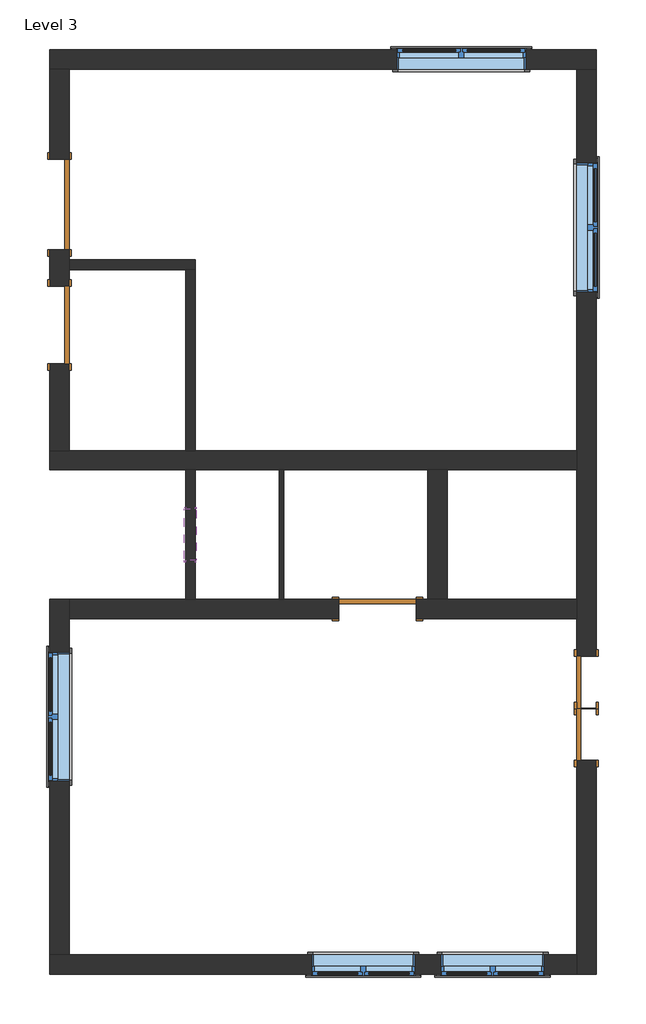
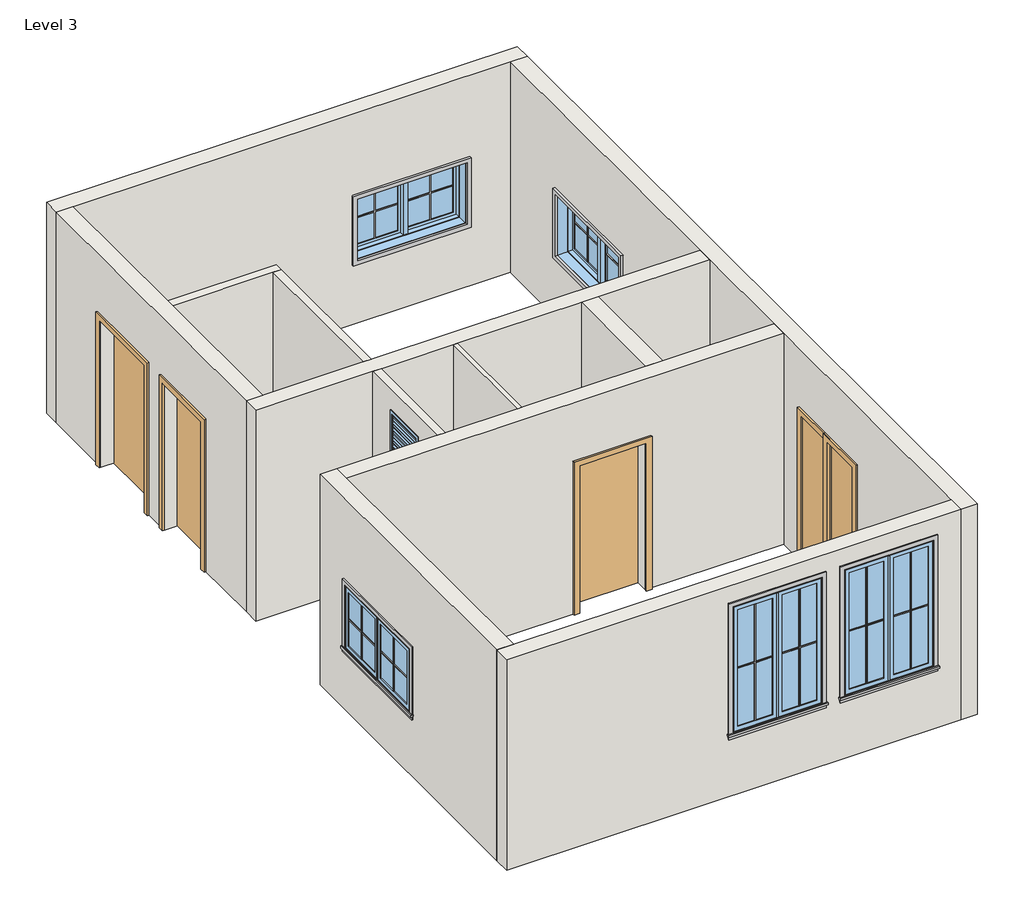
# One storey: 20 proxies, 12 walls, 6 windows, 5 doors.
"""IFC4 building model written with IfcOpenShell, lengths in millimetres."""

from ifc_helpers import new_model, si_unit, frame, origin, place, context, project, spatial, polyline, outline, extrude, faceted_brep, transform, mapped, element, save
from components import muntin_pattern_2x2_muntin_pattern_2x2_9352d081, muntin_pattern_2x2_muntin_pattern_2x2_5c2cbe28, muntin_pattern_2x2_muntin_pattern_2x2_2b4d9f72, muntin_pattern_2x2_muntin_pattern_2x2_ef995ed3, trim_window_exterior_flat_with_sill_979bde60, trim_window_exterior_flat_with_sill_b7e4d11c, trim_window_interior_flat_picture_frame_7883d11b, trim_window_interior_flat_picture_frame_936b8d2a, single_flush_door_2_0d3b4037, single_flush_door_2_4a3212df, door_a90ba1ad, door_0ca8825f, door_9d399b00, window_casement_double_c1d95f0f, window_casement_double_wall_4_6ca1769e, window_d39e7ecb

model = new_model("IFC4")

# Units and contexts
model_context = context("Model", 3, world=origin())
ifc_project = project(units=[si_unit("LENGTHUNIT", "METRE", prefix="MILLI")], contexts=[model_context])

# Site, building, storey
site = spatial("IfcSite", under=ifc_project)
building = spatial("IfcBuilding", under=site)
storey = spatial("IfcBuildingStorey", under=building, Name="Level 3", Elevation=3200.4)

# Proxies
placement = place(None, origin())
muntin_pattern_2x2_muntin_pattern_2x2_shape = muntin_pattern_2x2_muntin_pattern_2x2_9352d081(model_context)
element("IfcBuildingElementProxy", 1, Name="Muntin Pattern_2x2 : Muntin Pattern_2x2", ObjectType="Muntin Pattern_2x2 : Muntin Pattern_2x2", at=placement, inside=storey, context=model_context, shape_type="MappedRepresentation", body=[
    mapped(muntin_pattern_2x2_muntin_pattern_2x2_shape, transform((-4785.3510342, -2707.8617544, 4184.65), x_axis=(0.0, 1.0, 0.0), y_axis=(-1.0, 0.0, 0.0), z_axis=(0.0, 0.0, 1.0))),
])
element("IfcBuildingElementProxy", 2, Name="Muntin Pattern_2x2 : Muntin Pattern_2x2", ObjectType="Muntin Pattern_2x2 : Muntin Pattern_2x2", at=placement, inside=storey, context=model_context, shape_type="MappedRepresentation", body=[
    mapped(muntin_pattern_2x2_muntin_pattern_2x2_shape, transform((1634.4989658, 3816.7632456, 4184.65), x_axis=(0.0, -1.0, 0.0), y_axis=(1.0, 0.0, 0.0), z_axis=(0.0, 0.0, 1.0))),
])
element("IfcBuildingElementProxy", 3, Name="Muntin Pattern_2x2 : Muntin Pattern_2x2", ObjectType="Muntin Pattern_2x2 : Muntin Pattern_2x2", at=placement, inside=storey, context=model_context, shape_type="MappedRepresentation", body=[
    mapped(muntin_pattern_2x2_muntin_pattern_2x2_shape, transform((-322.8885342, 5523.3257456, 4184.65), x_axis=(1.0, 0.0, 0.0), y_axis=(0.0, 1.0, 0.0), z_axis=(0.0, 0.0, 1.0))),
])
muntin_pattern_2x2_muntin_pattern_2x2_2_shape = muntin_pattern_2x2_muntin_pattern_2x2_5c2cbe28(model_context)
element("IfcBuildingElementProxy", 4, Name="Muntin Pattern_2x2 : Muntin Pattern_2x2", ObjectType="Muntin Pattern_2x2 : Muntin Pattern_2x2", at=placement, inside=storey, context=model_context, shape_type="MappedRepresentation", body=[
    mapped(muntin_pattern_2x2_muntin_pattern_2x2_2_shape, transform((-4785.3510342, -1949.0367544, 4184.65), x_axis=(0.0, -1.0, 0.0), y_axis=(1.0, 0.0, 0.0), z_axis=(0.0, 0.0, 1.0))),
])
element("IfcBuildingElementProxy", 5, Name="Muntin Pattern_2x2 : Muntin Pattern_2x2", ObjectType="Muntin Pattern_2x2 : Muntin Pattern_2x2", at=placement, inside=storey, context=model_context, shape_type="MappedRepresentation", body=[
    mapped(muntin_pattern_2x2_muntin_pattern_2x2_2_shape, transform((1634.4989658, 3057.9382456, 4184.65), x_axis=(0.0, 1.0, 0.0), y_axis=(-1.0, 0.0, 0.0), z_axis=(0.0, 0.0, 1.0))),
])
element("IfcBuildingElementProxy", 6, Name="Muntin Pattern_2x2 : Muntin Pattern_2x2", ObjectType="Muntin Pattern_2x2 : Muntin Pattern_2x2", at=placement, inside=storey, context=model_context, shape_type="MappedRepresentation", body=[
    mapped(muntin_pattern_2x2_muntin_pattern_2x2_2_shape, transform((435.9364658, 5523.3257456, 4184.65), x_axis=(-1.0, 0.0, 0.0), y_axis=(0.0, -1.0, 0.0), z_axis=(0.0, 0.0, 1.0))),
])
muntin_pattern_2x2_muntin_pattern_2x2_3_shape = muntin_pattern_2x2_muntin_pattern_2x2_2b4d9f72(model_context)
element("IfcBuildingElementProxy", 7, Name="Muntin Pattern_2x2 : Muntin Pattern_2x2", ObjectType="Muntin Pattern_2x2 : Muntin Pattern_2x2", at=placement, inside=storey, context=model_context, shape_type="MappedRepresentation", body=[
    mapped(muntin_pattern_2x2_muntin_pattern_2x2_3_shape, transform((-795.9635342, -5354.2242544, 4184.65), x_axis=(-1.0, 0.0, 0.0), y_axis=(0.0, -1.0, 0.0), z_axis=(0.0, 0.0, 1.0))),
])
element("IfcBuildingElementProxy", 8, Name="Muntin Pattern_2x2 : Muntin Pattern_2x2", ObjectType="Muntin Pattern_2x2 : Muntin Pattern_2x2", at=placement, inside=storey, context=model_context, shape_type="MappedRepresentation", body=[
    mapped(muntin_pattern_2x2_muntin_pattern_2x2_3_shape, transform((728.0364658, -5354.2242544, 4184.65), x_axis=(-1.0, 0.0, 0.0), y_axis=(0.0, -1.0, 0.0), z_axis=(0.0, 0.0, 1.0))),
])
muntin_pattern_2x2_muntin_pattern_2x2_4_shape = muntin_pattern_2x2_muntin_pattern_2x2_ef995ed3(model_context)
element("IfcBuildingElementProxy", 9, Name="Muntin Pattern_2x2 : Muntin Pattern_2x2", ObjectType="Muntin Pattern_2x2 : Muntin Pattern_2x2", at=placement, inside=storey, context=model_context, shape_type="MappedRepresentation", body=[
    mapped(muntin_pattern_2x2_muntin_pattern_2x2_4_shape, transform((-1402.3885342, -5354.2242544, 4184.65), x_axis=(1.0, 0.0, 0.0), y_axis=(0.0, 1.0, 0.0), z_axis=(0.0, 0.0, 1.0))),
])
element("IfcBuildingElementProxy", 10, Name="Muntin Pattern_2x2 : Muntin Pattern_2x2", ObjectType="Muntin Pattern_2x2 : Muntin Pattern_2x2", at=placement, inside=storey, context=model_context, shape_type="MappedRepresentation", body=[
    mapped(muntin_pattern_2x2_muntin_pattern_2x2_4_shape, transform((121.6114658, -5354.2242544, 4184.65), x_axis=(1.0, 0.0, 0.0), y_axis=(0.0, 1.0, 0.0), z_axis=(0.0, 0.0, 1.0))),
])
trim_window_exterior_flat_with_sill_shape = trim_window_exterior_flat_with_sill_979bde60(model_context)
element("IfcBuildingElementProxy", 11, Name="Trim-Window-Exterior-Flat : with Sill", ObjectType="Trim-Window-Exterior-Flat : with Sill", at=placement, inside=storey, context=model_context, shape_type="MappedRepresentation", body=[
    mapped(trim_window_exterior_flat_with_sill_shape, transform((-4794.8760342, -2328.4492544, 5029.2), x_axis=(0.0, -1.0, 0.0), y_axis=(0.0, 0.0, 1.0), z_axis=(-1.0, 0.0, 0.0))),
])
element("IfcBuildingElementProxy", 12, Name="Trim-Window-Exterior-Flat : with Sill", ObjectType="Trim-Window-Exterior-Flat : with Sill", at=placement, inside=storey, context=model_context, shape_type="MappedRepresentation", body=[
    mapped(trim_window_exterior_flat_with_sill_shape, transform((1644.0239658, 3437.3507456, 5029.2), x_axis=(0.0, 1.0, 0.0), y_axis=(0.0, 0.0, 1.0), z_axis=(1.0, 0.0, 0.0))),
])
element("IfcBuildingElementProxy", 13, Name="Trim-Window-Exterior-Flat : with Sill", ObjectType="Trim-Window-Exterior-Flat : with Sill", at=placement, inside=storey, context=model_context, shape_type="MappedRepresentation", body=[
    mapped(trim_window_exterior_flat_with_sill_shape, transform((56.5239658, 5532.8507456, 5029.2), x_axis=(-1.0, 0.0, 0.0), y_axis=(0.0, 0.0, 1.0), z_axis=(0.0, 1.0, 0.0))),
])
trim_window_exterior_flat_with_sill_2_shape = trim_window_exterior_flat_with_sill_b7e4d11c(model_context)
element("IfcBuildingElementProxy", 14, Name="Trim-Window-Exterior-Flat : with Sill", ObjectType="Trim-Window-Exterior-Flat : with Sill", at=placement, inside=storey, context=model_context, shape_type="MappedRepresentation", body=[
    mapped(trim_window_exterior_flat_with_sill_2_shape, transform((-1099.1760342, -5363.7492544, 5943.6), x_axis=(1.0, 0.0, 0.0), y_axis=(0.0, 0.0, 1.0), z_axis=(0.0, -1.0, 0.0))),
])
element("IfcBuildingElementProxy", 15, Name="Trim-Window-Exterior-Flat : with Sill", ObjectType="Trim-Window-Exterior-Flat : with Sill", at=placement, inside=storey, context=model_context, shape_type="MappedRepresentation", body=[
    mapped(trim_window_exterior_flat_with_sill_2_shape, transform((424.8239658, -5363.7492544, 5943.6), x_axis=(1.0, 0.0, 0.0), y_axis=(0.0, 0.0, 1.0), z_axis=(0.0, -1.0, 0.0))),
])
trim_window_interior_flat_picture_frame_shape = trim_window_interior_flat_picture_frame_7883d11b(model_context)
element("IfcBuildingElementProxy", 16, Name="Trim-Window-Interior-Flat : Picture Frame", ObjectType="Trim-Window-Interior-Flat : Picture Frame", at=placement, inside=storey, context=model_context, shape_type="MappedRepresentation", body=[
    mapped(trim_window_interior_flat_picture_frame_shape, transform((-4566.2760342, -2328.4492544, 5029.2), x_axis=(0.0, 1.0, 0.0), y_axis=(0.0, 0.0, 1.0), z_axis=(1.0, 0.0, 0.0))),
])
element("IfcBuildingElementProxy", 17, Name="Trim-Window-Interior-Flat : Picture Frame", ObjectType="Trim-Window-Interior-Flat : Picture Frame", at=placement, inside=storey, context=model_context, shape_type="MappedRepresentation", body=[
    mapped(trim_window_interior_flat_picture_frame_shape, transform((1415.4239658, 3437.3507456, 5029.2), x_axis=(0.0, -1.0, 0.0), y_axis=(0.0, 0.0, 1.0), z_axis=(-1.0, 0.0, 0.0))),
])
element("IfcBuildingElementProxy", 18, Name="Trim-Window-Interior-Flat : Picture Frame", ObjectType="Trim-Window-Interior-Flat : Picture Frame", at=placement, inside=storey, context=model_context, shape_type="MappedRepresentation", body=[
    mapped(trim_window_interior_flat_picture_frame_shape, transform((56.5239658, 5304.2507456, 5029.2), x_axis=(1.0, 0.0, 0.0), y_axis=(0.0, 0.0, 1.0), z_axis=(0.0, -1.0, 0.0))),
])
trim_window_interior_flat_picture_frame_2_shape = trim_window_interior_flat_picture_frame_936b8d2a(model_context)
element("IfcBuildingElementProxy", 19, Name="Trim-Window-Interior-Flat : Picture Frame", ObjectType="Trim-Window-Interior-Flat : Picture Frame", at=placement, inside=storey, context=model_context, shape_type="MappedRepresentation", body=[
    mapped(trim_window_interior_flat_picture_frame_2_shape, transform((-1099.1760342, -5135.1492544, 5943.6), x_axis=(-1.0, 0.0, 0.0), y_axis=(0.0, 0.0, 1.0), z_axis=(0.0, 1.0, 0.0))),
])
element("IfcBuildingElementProxy", 20, Name="Trim-Window-Interior-Flat : Picture Frame", ObjectType="Trim-Window-Interior-Flat : Picture Frame", at=placement, inside=storey, context=model_context, shape_type="MappedRepresentation", body=[
    mapped(trim_window_interior_flat_picture_frame_2_shape, transform((424.8239658, -5135.1492544, 5943.6), x_axis=(-1.0, 0.0, 0.0), y_axis=(0.0, 0.0, 1.0), z_axis=(0.0, 1.0, 0.0))),
])

# Doors
single_flush_door_2_shape = single_flush_door_2_0d3b4037(model_context)
element("IfcDoor", 21, ObjectType="Single-Flush : door 2'", at=placement, inside=storey, context=model_context, shape_type="MappedRepresentation", body=[
    mapped(single_flush_door_2_shape, transform((1529.7239658, -1922.0492544, 3200.4), x_axis=(0.0, 1.0, 0.0), y_axis=(-1.0, 0.0, 0.0), z_axis=(0.0, 0.0, 1.0))),
])
single_flush_door_2_2_shape = single_flush_door_2_4a3212df(model_context)
element("IfcDoor", 22, ObjectType="Single-Flush : door 2'", at=placement, inside=storey, context=model_context, shape_type="MappedRepresentation", body=[
    mapped(single_flush_door_2_2_shape, transform((1529.7239658, -2537.9992544, 3200.4), x_axis=(0.0, -1.0, 0.0), y_axis=(1.0, 0.0, 0.0), z_axis=(0.0, 0.0, 1.0))),
])
door_shape = door_a90ba1ad(model_context)
element("IfcDoor", 23, ObjectType="Single-Flush : door 2'6\"", at=placement, inside=storey, context=model_context, shape_type="MappedRepresentation", body=[
    mapped(door_shape, transform((-4680.5760342, 2288.0007456, 3200.4), x_axis=(0.0, 1.0, 0.0), y_axis=(-1.0, 0.0, 0.0), z_axis=(0.0, 0.0, 1.0))),
])
door_2_shape = door_0ca8825f(model_context)
element("IfcDoor", 24, ObjectType="Single-Flush : door 2'6\"", at=placement, inside=storey, context=model_context, shape_type="MappedRepresentation", body=[
    mapped(door_2_shape, transform((-934.0760342, -1058.4492544, 3200.4), x_axis=(1.0, 0.0, 0.0), y_axis=(0.0, 1.0, 0.0), z_axis=(0.0, 0.0, 1.0))),
])
door_3_shape = door_9d399b00(model_context)
element("IfcDoor", 25, ObjectType="Single-Flush : door 3'6\"", at=placement, inside=storey, context=model_context, shape_type="MappedRepresentation", body=[
    mapped(door_3_shape, transform((-4680.5760342, 3710.4007456, 3200.4), x_axis=(0.0, -1.0, 0.0), y_axis=(1.0, 0.0, 0.0), z_axis=(0.0, 0.0, 1.0))),
])

# Walls
element("IfcWall", 26, ObjectType="wall 2\"", at=placement, inside=storey, context=model_context, shape_type="SweptSolid", body=[
    extrude(outline(polyline([(-2089.7760342, -944.1492544), (-2089.7760342, 579.8507456), (-2038.9760342, 579.8507456), (-2038.9760342, -944.1492544), (-2089.7760342, -944.1492544)])), frame((0.0, 0.0, 3200.4), z_axis=(0.0, 0.0, 1.0), x_axis=(1.0, 0.0, 0.0)), (0.0, 0.0, 1.0), 3048.0),
])
element("IfcWall", 27, ObjectType="wall 4.5\"", at=placement, inside=storey, context=model_context, shape_type="Brep", body=[
    faceted_brep([(-4566.2760342, 2942.0507456, 3200.4), (-3194.6760342, 2942.0507456, 3200.4), (-3080.3760342, 2942.0507456, 3200.4), (-3080.3760342, 2942.0507456, 6248.4), (-3194.6760342, 2942.0507456, 6248.4), (-4566.2760342, 2942.0507456, 6248.4), (-4566.2760342, 3056.3507456, 3200.4), (-4566.2760342, 3056.3507456, 6248.4), (-3080.3760342, 3056.3507456, 6248.4), (-3080.3760342, 3056.3507456, 3200.4)], [[[0, 1, 2, 3, 4, 5]], [[6, 7, 8, 9]], [[2, 1, 0, 6, 9]], [[0, 5, 7, 6]], [[3, 2, 9, 8]], [[5, 4, 3, 8, 7]]]),
])
element("IfcWall", 28, ObjectType="wall 4.5\"", at=placement, inside=storey, context=model_context, shape_type="SweptSolid", body=[
    extrude(outline(polyline([(-3194.6760342, 808.4507456), (-3194.6760342, 2942.0507456), (-3080.3760342, 2942.0507456), (-3080.3760342, 808.4507456), (-3194.6760342, 808.4507456)])), frame((0.0, 0.0, 3200.4), z_axis=(0.0, 0.0, 1.0), x_axis=(1.0, 0.0, 0.0)), (0.0, 0.0, 1.0), 3048.0),
])
element("IfcWall", 29, ObjectType="wall 4.5\"", at=placement, inside=storey, context=model_context, shape_type="SweptSolid", body=[
    extrude(outline(polyline([(579.8507456, 3200.4), (-944.1492544, 3200.4), (-944.1492544, 6248.4), (579.8507456, 6248.4), (579.8507456, 3200.4)]), holes=[polyline([(-486.9492544, 5943.6), (-486.9492544, 5334.0), (122.6507456, 5334.0), (122.6507456, 5943.6), (-486.9492544, 5943.6)])]), frame((-3194.6760342, 0.0, 0.0), z_axis=(1.0, 0.0, 0.0), x_axis=(0.0, 1.0, 0.0)), (0.0, 0.0, 1.0), 114.3),
])
element("IfcWall", 30, ObjectType="wall 9\"", at=placement, inside=storey, context=model_context, shape_type="Brep", body=[
    faceted_brep([(-4794.8760342, 5304.2507456, 3200.4), (-4566.2760342, 5304.2507456, 3200.4), (1415.4239658, 5304.2507456, 3200.4), (1644.0239658, 5304.2507456, 3200.4), (1644.0239658, 5304.2507456, 6248.4), (1415.4239658, 5304.2507456, 6248.4), (-4566.2760342, 5304.2507456, 6248.4), (-4794.8760342, 5304.2507456, 6248.4), (818.5239658, 5304.2507456, 5029.2), (818.5239658, 5304.2507456, 4114.8), (-705.4760342, 5304.2507456, 4114.8), (-705.4760342, 5304.2507456, 5029.2), (-4794.8760342, 5532.8507456, 3200.4), (-4794.8760342, 5532.8507456, 6248.4), (1644.0239658, 5532.8507456, 6248.4), (1644.0239658, 5532.8507456, 3200.4), (818.5239658, 5532.8507456, 5029.2), (-705.4760342, 5532.8507456, 5029.2), (-705.4760342, 5532.8507456, 4114.8), (818.5239658, 5532.8507456, 4114.8)], [[[0, 1, 2, 3, 4, 5, 6, 7], [8, 9, 10, 11]], [[12, 13, 14, 15], [16, 17, 18, 19]], [[3, 2, 1, 0, 12, 15]], [[4, 3, 15, 14]], [[0, 7, 13, 12]], [[9, 8, 16, 19]], [[10, 9, 19, 18]], [[11, 10, 18, 17]], [[8, 11, 17, 16]], [[7, 6, 5, 4, 14, 13]]]),
])
element("IfcWall", 31, ObjectType="wall 9\"", at=placement, inside=storey, context=model_context, shape_type="Brep", body=[
    faceted_brep([(1415.4239658, 5304.2507456, 6248.4), (1415.4239658, 5304.2507456, 3200.4), (1415.4239658, 808.4507456, 3200.4), (1415.4239658, 579.8507456, 3200.4), (1415.4239658, -944.1492544, 3200.4), (1415.4239658, -1172.7492544, 3200.4), (1415.4239658, -1617.2492544, 3200.4), (1415.4239658, -1617.2492544, 5334.0), (1415.4239658, -2226.8492544, 5334.0), (1415.4239658, -2226.8492544, 3200.4), (1415.4239658, -2233.1992544, 3200.4), (1415.4239658, -2233.1992544, 5334.0), (1415.4239658, -2842.7992544, 5334.0), (1415.4239658, -2842.7992544, 3200.4), (1415.4239658, -5135.1492544, 3200.4), (1415.4239658, -5363.7492544, 3200.4), (1415.4239658, -5363.7492544, 6248.4), (1415.4239658, -5135.1492544, 6248.4), (1415.4239658, -1172.7492544, 6248.4), (1415.4239658, -944.1492544, 6248.4), (1415.4239658, 579.8507456, 6248.4), (1415.4239658, 808.4507456, 6248.4), (1415.4239658, 2675.3507456, 5029.2), (1415.4239658, 2675.3507456, 4114.8), (1415.4239658, 4199.3507456, 4114.8), (1415.4239658, 4199.3507456, 5029.2), (1644.0239658, 5304.2507456, 3200.4), (1644.0239658, 5304.2507456, 6248.4), (1644.0239658, -5363.7492544, 6248.4), (1644.0239658, -5363.7492544, 3200.4), (1644.0239658, -2842.7992544, 3200.4), (1644.0239658, -2842.7992544, 5334.0), (1644.0239658, -2233.1992544, 5334.0), (1644.0239658, -2233.1992544, 3200.4), (1644.0239658, -2226.8492544, 3200.4), (1644.0239658, -2226.8492544, 5334.0), (1644.0239658, -1617.2492544, 5334.0), (1644.0239658, -1617.2492544, 3200.4), (1644.0239658, 2675.3507456, 5029.2), (1644.0239658, 4199.3507456, 5029.2), (1644.0239658, 4199.3507456, 4114.8), (1644.0239658, 2675.3507456, 4114.8)], [[[0, 1, 2, 3, 4, 5, 6, 7, 8, 9, 10, 11, 12, 13, 14, 15, 16, 17, 18, 19, 20, 21], [22, 23, 24, 25]], [[26, 27, 28, 29, 30, 31, 32, 33, 34, 35, 36, 37], [38, 39, 40, 41]], [[1, 26, 37, 6, 5, 4, 3, 2]], [[29, 15, 14, 13, 30]], [[9, 34, 33, 10]], [[1, 0, 27, 26]], [[16, 15, 29, 28]], [[23, 22, 38, 41]], [[24, 23, 41, 40]], [[25, 24, 40, 39]], [[22, 25, 39, 38]], [[7, 6, 37, 36]], [[8, 7, 36, 35]], [[9, 8, 35, 34]], [[12, 31, 30, 13]], [[31, 12, 11, 32]], [[32, 11, 10, 33]], [[0, 21, 20, 19, 18, 17, 16, 28, 27]]]),
])
element("IfcWall", 32, ObjectType="wall 9\"", at=placement, inside=storey, context=model_context, shape_type="Brep", body=[
    faceted_brep([(1415.4239658, 808.4507456, 3200.4), (-3080.3760342, 808.4507456, 3200.4), (-3194.6760342, 808.4507456, 3200.4), (-4566.2760342, 808.4507456, 3200.4), (-4794.8760342, 808.4507456, 3200.4), (-4794.8760342, 808.4507456, 6248.4), (-4566.2760342, 808.4507456, 6248.4), (-3194.6760342, 808.4507456, 6248.4), (-3080.3760342, 808.4507456, 6248.4), (1415.4239658, 808.4507456, 6248.4), (1415.4239658, 579.8507456, 3200.4), (1415.4239658, 579.8507456, 6248.4), (-108.5760342, 579.8507456, 6248.4), (-337.1760342, 579.8507456, 6248.4), (-2038.9760342, 579.8507456, 6248.4), (-2089.7760342, 579.8507456, 6248.4), (-3080.3760342, 579.8507456, 6248.4), (-3194.6760342, 579.8507456, 6248.4), (-4794.8760342, 579.8507456, 6248.4), (-4794.8760342, 579.8507456, 3200.4), (-3194.6760342, 579.8507456, 3200.4), (-3080.3760342, 579.8507456, 3200.4), (-2089.7760342, 579.8507456, 3200.4), (-2038.9760342, 579.8507456, 3200.4), (-337.1760342, 579.8507456, 3200.4), (-108.5760342, 579.8507456, 3200.4)], [[[0, 1, 2, 3, 4, 5, 6, 7, 8, 9]], [[10, 11, 12, 13, 14, 15, 16, 17, 18, 19, 20, 21, 22, 23, 24, 25]], [[4, 3, 2, 1, 0, 10, 25, 24, 23, 22, 21, 20, 19]], [[0, 9, 11, 10]], [[5, 4, 19, 18]], [[9, 8, 7, 6, 5, 18, 17, 16, 15, 14, 13, 12, 11]]]),
])
element("IfcWall", 33, ObjectType="wall 9\"", at=placement, inside=storey, context=model_context, shape_type="Brep", body=[
    faceted_brep([(-4566.2760342, 2745.2007456, 5334.0), (-4566.2760342, 2745.2007456, 3200.4), (-4566.2760342, 2942.0507456, 3200.4), (-4566.2760342, 3056.3507456, 3200.4), (-4566.2760342, 3177.0007456, 3200.4), (-4566.2760342, 3177.0007456, 5334.0), (-4566.2760342, 4243.8007456, 5334.0), (-4566.2760342, 4243.8007456, 3200.4), (-4566.2760342, 5304.2507456, 3200.4), (-4566.2760342, 5304.2507456, 6248.4), (-4566.2760342, 3056.3507456, 6248.4), (-4566.2760342, 2942.0507456, 6248.4), (-4566.2760342, 808.4507456, 6248.4), (-4566.2760342, 808.4507456, 3200.4), (-4566.2760342, 1830.8007456, 3200.4), (-4566.2760342, 1830.8007456, 5334.0), (-4794.8760342, 3177.0007456, 3200.4), (-4794.8760342, 2745.2007456, 3200.4), (-4794.8760342, 2745.2007456, 5334.0), (-4794.8760342, 1830.8007456, 5334.0), (-4794.8760342, 1830.8007456, 3200.4), (-4794.8760342, 808.4507456, 3200.4), (-4794.8760342, 808.4507456, 6248.4), (-4794.8760342, 5304.2507456, 6248.4), (-4794.8760342, 5304.2507456, 3200.4), (-4794.8760342, 4243.8007456, 3200.4), (-4794.8760342, 4243.8007456, 5334.0), (-4794.8760342, 3177.0007456, 5334.0)], [[[0, 1, 2, 3, 4, 5, 6, 7, 8, 9, 10, 11, 12, 13, 14, 15]], [[16, 17, 18, 19, 20, 21, 22, 23, 24, 25, 26, 27]], [[25, 24, 8, 7]], [[14, 13, 21, 20]], [[4, 3, 2, 1, 17, 16]], [[9, 8, 24, 23]], [[13, 12, 22, 21]], [[5, 4, 16, 27]], [[6, 5, 27, 26]], [[7, 6, 26, 25]], [[18, 17, 1, 0]], [[19, 18, 0, 15]], [[20, 19, 15, 14]], [[12, 11, 10, 9, 23, 22]]]),
])
element("IfcWall", 34, ObjectType="wall 9\"", at=placement, inside=storey, context=model_context, shape_type="Brep", body=[
    faceted_brep([(1415.4239658, -5135.1492544, 3200.4), (-4566.2760342, -5135.1492544, 3200.4), (-4794.8760342, -5135.1492544, 3200.4), (-4794.8760342, -5135.1492544, 6248.4), (-4566.2760342, -5135.1492544, 6248.4), (1415.4239658, -5135.1492544, 6248.4), (-1708.7760342, -5135.1492544, 5943.6), (-1708.7760342, -5135.1492544, 4114.8), (-489.5760342, -5135.1492544, 4114.8), (-489.5760342, -5135.1492544, 5943.6), (-184.7760342, -5135.1492544, 5943.6), (-184.7760342, -5135.1492544, 4114.8), (1034.4239658, -5135.1492544, 4114.8), (1034.4239658, -5135.1492544, 5943.6), (1415.4239658, -5363.7492544, 3200.4), (1415.4239658, -5363.7492544, 6248.4), (-4794.8760342, -5363.7492544, 6248.4), (-4794.8760342, -5363.7492544, 3200.4), (-1708.7760342, -5363.7492544, 5943.6), (-489.5760342, -5363.7492544, 5943.6), (-489.5760342, -5363.7492544, 4114.8), (-1708.7760342, -5363.7492544, 4114.8), (-184.7760342, -5363.7492544, 5943.6), (1034.4239658, -5363.7492544, 5943.6), (1034.4239658, -5363.7492544, 4114.8), (-184.7760342, -5363.7492544, 4114.8)], [[[0, 1, 2, 3, 4, 5], [6, 7, 8, 9], [10, 11, 12, 13]], [[14, 15, 16, 17], [18, 19, 20, 21], [22, 23, 24, 25]], [[2, 1, 0, 14, 17]], [[0, 5, 15, 14]], [[3, 2, 17, 16]], [[7, 6, 18, 21]], [[8, 7, 21, 20]], [[9, 8, 20, 19]], [[6, 9, 19, 18]], [[11, 10, 22, 25]], [[12, 11, 25, 24]], [[13, 12, 24, 23]], [[10, 13, 23, 22]], [[5, 4, 3, 16, 15]]]),
])
element("IfcWall", 35, ObjectType="wall 9\"", at=placement, inside=storey, context=model_context, shape_type="Brep", body=[
    faceted_brep([(-4566.2760342, -5135.1492544, 3200.4), (-4566.2760342, -1172.7492544, 3200.4), (-4566.2760342, -944.1492544, 3200.4), (-4566.2760342, -944.1492544, 6248.4), (-4566.2760342, -1172.7492544, 6248.4), (-4566.2760342, -5135.1492544, 6248.4), (-4566.2760342, -1566.4492544, 5029.2), (-4566.2760342, -1566.4492544, 4114.8), (-4566.2760342, -3090.4492544, 4114.8), (-4566.2760342, -3090.4492544, 5029.2), (-4794.8760342, -5135.1492544, 3200.4), (-4794.8760342, -5135.1492544, 6248.4), (-4794.8760342, -944.1492544, 6248.4), (-4794.8760342, -944.1492544, 3200.4), (-4794.8760342, -1566.4492544, 5029.2), (-4794.8760342, -3090.4492544, 5029.2), (-4794.8760342, -3090.4492544, 4114.8), (-4794.8760342, -1566.4492544, 4114.8)], [[[0, 1, 2, 3, 4, 5], [6, 7, 8, 9]], [[10, 11, 12, 13], [14, 15, 16, 17]], [[2, 1, 0, 10, 13]], [[0, 5, 11, 10]], [[3, 2, 13, 12]], [[7, 6, 14, 17]], [[8, 7, 17, 16]], [[9, 8, 16, 15]], [[6, 9, 15, 14]], [[5, 4, 3, 12, 11]]]),
])
element("IfcWall", 36, ObjectType="wall 9\"", at=placement, inside=storey, context=model_context, shape_type="Brep", body=[
    faceted_brep([(-476.8760342, -1172.7492544, 5334.0), (-476.8760342, -1172.7492544, 3200.4), (1415.4239658, -1172.7492544, 3200.4), (1415.4239658, -1172.7492544, 6248.4), (-4566.2760342, -1172.7492544, 6248.4), (-4566.2760342, -1172.7492544, 3200.4), (-1391.2760342, -1172.7492544, 3200.4), (-1391.2760342, -1172.7492544, 5334.0), (1415.4239658, -944.1492544, 3200.4), (-108.5760342, -944.1492544, 3200.4), (-337.1760342, -944.1492544, 3200.4), (-476.8760342, -944.1492544, 3200.4), (-476.8760342, -944.1492544, 5334.0), (-1391.2760342, -944.1492544, 5334.0), (-1391.2760342, -944.1492544, 3200.4), (-2038.9760342, -944.1492544, 3200.4), (-2089.7760342, -944.1492544, 3200.4), (-3080.3760342, -944.1492544, 3200.4), (-3194.6760342, -944.1492544, 3200.4), (-4566.2760342, -944.1492544, 3200.4), (-4566.2760342, -944.1492544, 6248.4), (-3194.6760342, -944.1492544, 6248.4), (-3080.3760342, -944.1492544, 6248.4), (-2089.7760342, -944.1492544, 6248.4), (-2038.9760342, -944.1492544, 6248.4), (-337.1760342, -944.1492544, 6248.4), (-108.5760342, -944.1492544, 6248.4), (1415.4239658, -944.1492544, 6248.4)], [[[0, 1, 2, 3, 4, 5, 6, 7]], [[8, 9, 10, 11, 12, 13, 14, 15, 16, 17, 18, 19, 20, 21, 22, 23, 24, 25, 26, 27]], [[6, 5, 19, 18, 17, 16, 15, 14]], [[2, 1, 11, 10, 9, 8]], [[5, 4, 20, 19]], [[3, 2, 8, 27]], [[12, 11, 1, 0]], [[13, 12, 0, 7]], [[14, 13, 7, 6]], [[4, 3, 27, 26, 25, 24, 23, 22, 21, 20]]]),
])
element("IfcWall", 37, ObjectType="wall 9\"", at=placement, inside=storey, context=model_context, shape_type="SweptSolid", body=[
    extrude(outline(polyline([(-108.5760342, 579.8507456), (-108.5760342, -944.1492544), (-337.1760342, -944.1492544), (-337.1760342, 579.8507456), (-108.5760342, 579.8507456)])), frame((0.0, 0.0, 3200.4), z_axis=(0.0, 0.0, 1.0), x_axis=(1.0, 0.0, 0.0)), (0.0, 0.0, 1.0), 3048.0),
])

# Windows
window_casement_double_shape = window_casement_double_c1d95f0f(model_context)
element("IfcWindow", 38, ObjectType="Window-Casement-Double", at=placement, inside=storey, context=model_context, shape_type="MappedRepresentation", body=[
    mapped(window_casement_double_shape, transform((-4680.5760342, -2328.4492544, 3200.4), x_axis=(0.0, 1.0, 0.0), y_axis=(-1.0, 0.0, 0.0), z_axis=(0.0, 0.0, 1.0))),
])
element("IfcWindow", 39, ObjectType="Window-Casement-Double", at=placement, inside=storey, context=model_context, shape_type="MappedRepresentation", body=[
    mapped(window_casement_double_shape, transform((1529.7239658, 3437.3507456, 3200.4), x_axis=(0.0, -1.0, 0.0), y_axis=(1.0, 0.0, 0.0), z_axis=(0.0, 0.0, 1.0))),
])
element("IfcWindow", 40, ObjectType="Window-Casement-Double", at=placement, inside=storey, context=model_context, shape_type="MappedRepresentation", body=[
    mapped(window_casement_double_shape, transform((56.5239658, 5418.5507456, 3200.4), x_axis=(1.0, 0.0, 0.0), y_axis=(0.0, 1.0, 0.0), z_axis=(0.0, 0.0, 1.0))),
])
window_casement_double_wall_4_shape = window_casement_double_wall_4_6ca1769e(model_context)
element("IfcWindow", 41, ObjectType="Window-Casement-Double : wall 4'", at=placement, inside=storey, context=model_context, shape_type="MappedRepresentation", body=[
    mapped(window_casement_double_wall_4_shape, transform((-1099.1760342, -5249.4492544, 3200.4), x_axis=(-1.0, 0.0, 0.0), y_axis=(0.0, -1.0, 0.0), z_axis=(0.0, 0.0, 1.0))),
])
element("IfcWindow", 42, ObjectType="Window-Casement-Double : wall 4'", at=placement, inside=storey, context=model_context, shape_type="MappedRepresentation", body=[
    mapped(window_casement_double_wall_4_shape, transform((424.8239658, -5249.4492544, 3200.4), x_axis=(-1.0, 0.0, 0.0), y_axis=(0.0, -1.0, 0.0), z_axis=(0.0, 0.0, 1.0))),
])
window_shape = window_d39e7ecb(model_context)
element("IfcWindow", 43, ObjectType="Window-Louvers : 24\" x 24\"", at=placement, inside=storey, context=model_context, shape_type="MappedRepresentation", body=[
    mapped(window_shape, transform((-3143.8760342, -182.1492544, 4419.6), x_axis=(0.0, 1.0, 0.0), y_axis=(-1.0, 0.0, 0.0), z_axis=(0.0, 0.0, 1.0))),
])

save(model, "model.ifc")

# Revit data of these elements
# Type "Muntin Pattern_2x2 : Muntin Pattern_2x2"
#   Width [instance default] = 4' - 0"
#   Thickness = 0' - 0 1/2"
#   Height [instance default] = 4' - 0"
#   Distance = 0' - 0 3/4"
#   Interior Material [instance default] = none
#   Exterior Material [instance default] = none
#   Default Elevation = 0
# Type "Trim-Window-Exterior-Flat : with Sill"
#   Trim Width = 0' - 2 1/4"
#   Trim Thickness_Picture Frame = 0' - 1 1/4"
#   Trim Thickness_with Sill = 0' - 0 3/4"
#   Sill Thickness = 0' - 1 1/4"
#   Opening Width [instance default] = 2' - 0"
#   Opening Height [instance default] = 3' - 0"
#   Default Elevation = 4' - 0"
#   Sill = yes
#   Picture Frame = no
#   Trim Material [instance default] = none
# Type "Trim-Window-Interior-Flat : Picture Frame"
#   Trim Thickness_Picture Frame = 0' - 1 1/4"
#   Trim Width = 0' - 2 1/4"
#   Trim Thickness_with Sill = 0' - 0 3/4"
#   Sill Thickness = 0' - 1 1/4"
#   Opening Width [instance default] = 2' - 0"
#   Opening Height [instance default] = 3' - 0"
#   Default Elevation = 4' - 0"
#   Sill = no
#   Picture Frame = yes
#   Trim Material [instance default] = none
# Type "Single-Flush : door 2'"
#   Type Mark = "11"
#   Construction Type Id = "MDOOR"
#   Assembly Code = "C1020"
#   Analytic Construction = "Metal"
#   Thickness = 0' - 2"
#   Heat Transfer Coefficient (U) = 0.651978 BTU/(h·ft²·°F)
#   Height = 7' - 0"
#   Trim Projection Ext = 0' - 1"
#   Trim Projection Int = 0' - 1"
#   Trim Width = 0' - 3"
#   Width = 2' - 0"
#   Define Thermal Properties by = 1
#   Door Material = Door - Panel
#   Frame Material = Door - Frame
#   Visual Light Transmittance = 0
#   Solar Heat Gain Coefficient = 0
#   Function = (empty or 0)
#   Wall Closure = (empty or 0)
# Type "Single-Flush : door 2'6\""
#   Type Mark = "8"
#   Construction Type Id = "MDOOR"
#   Assembly Code = "C1020"
#   Analytic Construction = "Metal"
#   Thickness = 0' - 2"
#   Heat Transfer Coefficient (U) = 0.651978 BTU/(h·ft²·°F)
#   Height = 7' - 0"
#   Trim Projection Ext = 0' - 1"
#   Trim Projection Int = 0' - 1"
#   Trim Width = 0' - 3"
#   Width = 3' - 0"
#   Define Thermal Properties by = 1
#   Door Material = Door - Panel
#   Frame Material = Door - Frame
#   Visual Light Transmittance = 0
#   Solar Heat Gain Coefficient = 0
#   Function = (empty or 0)
#   Wall Closure = (empty or 0)
# Type "Single-Flush : door 3'6\""
#   Type Mark = "10"
#   Construction Type Id = "MDOOR"
#   Assembly Code = "C1020"
#   Analytic Construction = "Metal"
#   Thickness = 0' - 2"
#   Heat Transfer Coefficient (U) = 0.651978 BTU/(h·ft²·°F)
#   Height = 7' - 0"
#   Trim Projection Ext = 0' - 1"
#   Trim Projection Int = 0' - 1"
#   Trim Width = 0' - 3"
#   Width = 3' - 6"
#   Define Thermal Properties by = 1
#   Door Material = Door - Panel
#   Frame Material = Door - Frame
#   Visual Light Transmittance = 0
#   Solar Heat Gain Coefficient = 0
#   Function = (empty or 0)
#   Wall Closure = (empty or 0)
# Type "wall 2\""
#   Assembly Code = "B2010"
#   Layers, outside or top first: 0' - 2" no material (function 1)
# Type "wall 4.5\""
#   Assembly Code = "B2010"
#   Layers, outside or top first: 0' - 4 1/2" no material (function 1)
# Type "wall 9\""
#   Assembly Code = "B2010"
#   Layers, outside or top first: 0' - 9" no material (function 1)
# Type "Window-Casement-Double"
#   Type Mark = "18"
#   Fire Rating = "0.5h"
#   Assembly Code = "B2020100"
#   Analytic Construction = "Double glazing - domestic"
#   Frame Extension [instance default] = 0' - 0 1/4"
#   Window Inset [instance default] = 0' - 0"
#   Wall Thickness [instance default] = 0' - 6"
#   Interior Wall Closure [instance default] = 0' - 2 1/4"
#   Half Width = 2' - 6"
#   Visual Light Transmittance = 0.81
#   Thermal Resistance (R) = 1.8146 (h·ft²·°F)/BTU
#   Solar Heat Gain Coefficient = 0.76
#   Rough Width = 5' - 0 1/2"
#   Rough Height = 3' - 0 1/2"
#   Height = 3' - 0"
#   Heat Transfer Coefficient (U) = 0.5511 BTU/(h·ft²·°F)
#   Exterior Wall Closure [instance default] = 0' - 1 1/4"
#   Extension Jamb [instance default] = 0' - 2 1/4"
#   Default Sill Height = 3' - 0"
#   Width = 5' - 0"
#   Muntin Visibility = yes
#   Interior Trim Visibility [instance default] = yes
#   Exterior Trim Visibility [instance default] = yes
#   Extension Jamb Visibility [instance default] = yes
#   Interior Trim Material = Wood - Stained
#   Muntin Pattern = Muntin Pattern_2x2 : Muntin Pattern_2x2
#   Interior Trim = Trim-Window-Interior-Flat : Picture Frame
#   Interior Frame Material = Wood - Stained
#   Glass Panel Material = Glass
#   Exterior Trim Material = Clad - White
#   Exterior Trim = Trim-Window-Exterior-Flat : with Sill
#   Exterior Frame Material = Clad - White
#   Wall Closure = (empty or 0)
# Type "Window-Casement-Double : wall 4'"
#   Type Mark = "19"
#   Fire Rating = "0.5h"
#   Assembly Code = "B2020100"
#   Analytic Construction = "Double glazing - domestic"
#   Frame Extension [instance default] = 0' - 0 1/4"
#   Window Inset [instance default] = 0' - 0"
#   Wall Thickness [instance default] = 0' - 6"
#   Interior Wall Closure [instance default] = 0' - 2 1/4"
#   Half Width = 2' - 0"
#   Visual Light Transmittance = 0.81
#   Thermal Resistance (R) = 1.8146 (h·ft²·°F)/BTU
#   Solar Heat Gain Coefficient = 0.76
#   Rough Width = 4' - 0 1/2"
#   Rough Height = 6' - 0 1/2"
#   Height = 6' - 0"
#   Heat Transfer Coefficient (U) = 0.5511 BTU/(h·ft²·°F)
#   Exterior Wall Closure [instance default] = 0' - 1 1/4"
#   Extension Jamb [instance default] = 0' - 2 1/4"
#   Default Sill Height = 3' - 0"
#   Width = 4' - 0"
#   Muntin Visibility = yes
#   Interior Trim Visibility [instance default] = yes
#   Exterior Trim Visibility [instance default] = yes
#   Extension Jamb Visibility [instance default] = yes
#   Interior Trim Material = Wood - Stained
#   Muntin Pattern = Muntin Pattern_2x2 : Muntin Pattern_2x2
#   Interior Trim = Trim-Window-Interior-Flat : Picture Frame
#   Interior Frame Material = Wood - Stained
#   Glass Panel Material = Glass
#   Exterior Trim Material = Clad - White
#   Exterior Trim = Trim-Window-Exterior-Flat : with Sill
#   Exterior Frame Material = Clad - White
#   Wall Closure = (empty or 0)
# Type "Window-Louvers : 24\" x 24\""
#   Type Mark = "20"
#   Construction Type Id = "GSP4R"
#   Assembly Code = "B20"
#   Analytic Construction = "1/8 in Pilkington single glazing"
#   Visual Light Transmittance = 0.9
#   Thermal Resistance (R) = 1.53941 (h·ft²·°F)/BTU
#   Solar Heat Gain Coefficient = 0.78
#   Max Height = 1' - 11.74264"
#   Height = 2' - 0"
#   Heat Transfer Coefficient (U) = 0.6496 BTU/(h·ft²·°F)
#   Blade Width [instance default] = 1' - 10 1/2"
#   Blade Vertical Thickness = 0' - 0.35355"
#   Blade Thickness = 0' - 0 1/4"
#   Blade Spacing = 0' - 1 1/2"
#   Blade Height = 0' - 1.85355"
#   Blade Depth = 0' - 3"
#   Blade Angle = 45.00°
#   Default Sill Height = 3' - 0"
#   Trim Projection_Exterior = 0' - 0 1/2"
#   Trim Projection_Interior = 0' - 0 1/2"
#   Trim Width_Exterior = 0' - 1 1/2"
#   Trim Width_Interior = 0' - 1 1/2"
#   Width = 2' - 0"
#   Max Blade Count = 12
#   Define Thermal Properties by = 1
#   Blade Count = 12
#   Frame Material = Birch
#   Louver Material = Birch
#   Trim Exterior Material = Birch
#   Trim Interior Material = Birch
#   Wall Closure = (empty or 0)
# Elements 1, 2, 3, 4, 5, 6 (IfcBuildingElementProxy, "Muntin Pattern_2x2 : Muntin Pattern_2x2")
#   Width = 2' - 0 5/8"
#   Height = 2' - 6 1/2"
#   Interior Material = Wood - Stained
#   Exterior Material = Clad - White
#   Phase Created = New Construction
#   Materials on its faces: "Clad - White", "Wood - Stained"
# Elements 7, 8, 9, 10 (IfcBuildingElementProxy, "Muntin Pattern_2x2 : Muntin Pattern_2x2")
#   Width = 1' - 6 5/8"
#   Height = 5' - 6 1/2"
#   Interior Material = Wood - Stained
#   Exterior Material = Clad - White
#   Phase Created = New Construction
#   Materials on its faces: "Clad - White", "Wood - Stained"
# Elements 11, 12, 13 (IfcBuildingElementProxy, "Trim-Window-Exterior-Flat : with Sill")
#   Opening Width = 5' - 0"
#   Opening Height = 3' - 0"
#   Trim Material = Clad - White
#   Phase Created = New Construction
#   Materials on its faces: "Clad - White"
# Elements 14, 15 (IfcBuildingElementProxy, "Trim-Window-Exterior-Flat : with Sill")
#   Opening Width = 4' - 0"
#   Opening Height = 6' - 0"
#   Trim Material = Clad - White
#   Phase Created = New Construction
#   Materials on its faces: "Clad - White"
# Elements 16, 17, 18 (IfcBuildingElementProxy, "Trim-Window-Interior-Flat : Picture Frame")
#   Opening Width = 5' - 0"
#   Opening Height = 3' - 0"
#   Trim Material = Wood - Stained
#   Phase Created = New Construction
#   Materials on its faces: "Wood - Stained"
# Elements 19, 20 (IfcBuildingElementProxy, "Trim-Window-Interior-Flat : Picture Frame")
#   Opening Width = 4' - 0"
#   Opening Height = 6' - 0"
#   Trim Material = Wood - Stained
#   Phase Created = New Construction
#   Materials on its faces: "Wood - Stained"
# Elements 21, 22 (IfcDoor, "Single-Flush : door 2'")
#   Phase Created = New Construction
#   Materials on its faces: "Door - Frame", "Door - Panel"
# Elements 23, 24 (IfcDoor, "Single-Flush : door 2'6\"")
#   Phase Created = New Construction
#   Materials on its faces: "Door - Frame", "Door - Panel"
# Element 25 (IfcDoor, "Single-Flush : door 3'6\"")
#   Phase Created = New Construction
#   Materials on its faces: "Door - Frame", "Door - Panel"
# Element 26 (IfcWall, "wall 2\"")
#   Top Offset = 0' - 0"
#   Base Offset = 0' - 0"
#   Unconnected Height = 10' - 0"
#   wall height = 10' - 0"
#   Phase Created = New Construction
#   Base Constraint = Level 3
#   Materials on its faces: "Default Wall"
# Elements 27, 28 (IfcWall, "wall 4.5\"")
#   Top Offset = 0' - 0"
#   Base Offset = 0' - 0"
#   Unconnected Height = 10' - 0"
#   wall height = 10' - 0"
#   Phase Created = New Construction
#   Base Constraint = Level 3
#   Materials on its faces: "Default Wall"
# Element 29 (IfcWall, "wall 4.5\"")
#   Top Offset = 0' - 0"
#   Base Offset = 0' - 0"
#   Unconnected Height = 10' - 0"
#   wall height = 10' - 0"
#   Phase Created = New Construction
#   Base Constraint = Level 3
#   Materials on its faces: "Default Wall", "Wood Planks"
# Elements 30, 31, 32, 34, 35, 36 (IfcWall, "wall 9\"")
#   Top Offset = 0' - 0"
#   Base Offset = 0' - 0"
#   Unconnected Height = 10' - 0"
#   wall height = 10' - 0"
#   Phase Created = New Construction
#   Base Constraint = Level 3
#   Materials on its faces: "Default Wall", "Wood Planks"
# Element 33 (IfcWall, "wall 9\"")
#   Top Offset = 0' - 0"
#   Base Offset = 0' - 0"
#   Unconnected Height = 10' - 0"
#   wall height = 10' - 0"
#   Phase Created = New Construction
#   Base Constraint = Level 3
#   Materials on its faces: "Default Wall", "Copper", "Wood Planks"
# Element 37 (IfcWall, "wall 9\"")
#   Top Offset = 0' - 0"
#   Base Offset = 0' - 0"
#   Unconnected Height = 10' - 0"
#   wall height = 10' - 0"
#   Phase Created = New Construction
#   Base Constraint = Level 3
#   Materials on its faces: "Default Wall"
# Element 38 (IfcWindow, "Window-Casement-Double")
#   Mark = "7"
#   Window Inset = 0' - 0"
#   Interior Wall Closure = 0' - 2 1/4"
#   Frame Extension = 0' - 0 1/4"
#   Exterior Wall Closure = 0' - 1 1/4"
#   Interior Trim Visibility = yes
#   Exterior Trim Visibility = yes
#   Phase Created = New Construction
#   Materials on its faces: "Wood - Stained", "Glass", "Clad - White"
# Element 39 (IfcWindow, "Window-Casement-Double")
#   Mark = "8"
#   Window Inset = 0' - 0"
#   Interior Wall Closure = 0' - 2 1/4"
#   Frame Extension = 0' - 0 1/4"
#   Exterior Wall Closure = 0' - 1 1/4"
#   Interior Trim Visibility = yes
#   Exterior Trim Visibility = yes
#   Phase Created = New Construction
#   Materials on its faces: "Wood - Stained", "Glass", "Clad - White"
# Element 40 (IfcWindow, "Window-Casement-Double")
#   Mark = "9"
#   Window Inset = 0' - 0"
#   Interior Wall Closure = 0' - 2 1/4"
#   Frame Extension = 0' - 0 1/4"
#   Exterior Wall Closure = 0' - 1 1/4"
#   Interior Trim Visibility = yes
#   Exterior Trim Visibility = yes
#   Phase Created = New Construction
#   Materials on its faces: "Wood - Stained", "Glass", "Clad - White"
# Element 41 (IfcWindow, "Window-Casement-Double : wall 4'")
#   Mark = "10"
#   Window Inset = 0' - 0"
#   Interior Wall Closure = 0' - 2 1/4"
#   Frame Extension = 0' - 0 1/4"
#   Exterior Wall Closure = 0' - 1 1/4"
#   Interior Trim Visibility = yes
#   Exterior Trim Visibility = yes
#   Phase Created = New Construction
#   Materials on its faces: "Wood - Stained", "Glass", "Clad - White"
# Element 42 (IfcWindow, "Window-Casement-Double : wall 4'")
#   Mark = "11"
#   Window Inset = 0' - 0"
#   Interior Wall Closure = 0' - 2 1/4"
#   Frame Extension = 0' - 0 1/4"
#   Exterior Wall Closure = 0' - 1 1/4"
#   Interior Trim Visibility = yes
#   Exterior Trim Visibility = yes
#   Phase Created = New Construction
#   Materials on its faces: "Wood - Stained", "Glass", "Clad - White"
# Element 43 (IfcWindow, "Window-Louvers : 24\" x 24\"")
#   Mark = "12"
#   Blade Width = 1' - 10 1/2"
#   Phase Created = New Construction
#   Materials on its faces: "Birch"
# Materials
#   "Door - Panel": class "Wood", colour RGB 210 159 95, transparency 0, Cost = 0
#   "Door - Frame": colour RGB 118 70 51, transparency 0, Cost = 0
#   "Wood - Stained": class "Wood", colour RGB 224 178 126, transparency 0, Cost = 0
#   "Glass": class "Glass", colour RGB 0 128 192, transparency 0.75, Description = "Soda Lime Glass", Cost = 0
#   "Clad - White": class "Wood", colour RGB 242 242 238, transparency 0, Cost = 0
#   "Birch": class "Wood", colour RGB 224 178 126, transparency 0, Description = "Betula Alleghaniensis", Cost = 0
#   "Default Wall": colour RGB 128 128 128, transparency 0, Cost = 0
#   "Wood Planks": class "Wood", colour RGB 193 160 115, transparency 0, Description = "Physical material.", Cost = 0
#   "Copper": class "Metal", colour RGB 0 0 0, transparency 0, Description = "Copper, matte finish", Cost = 0
